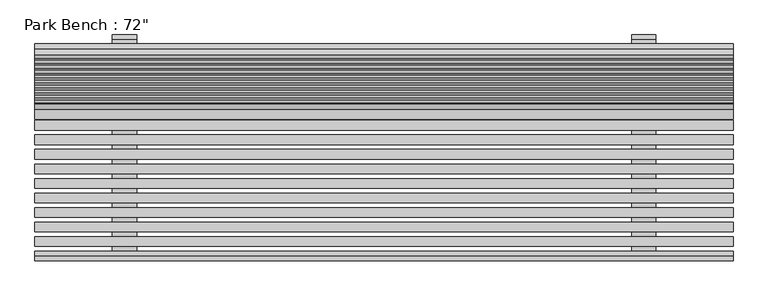
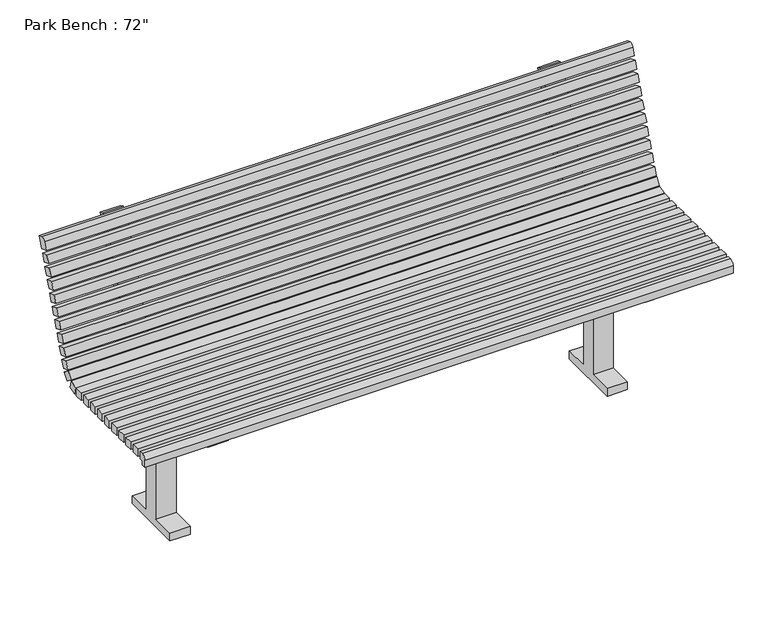
"""IFC4 building model written with IfcOpenShell, lengths in millimetres: geographic element geometry."""

from ifc_helpers import new_model, si_unit, point, frame, frame_2d, origin, place, context, project, spatial, polyline, circle_curve, trimmed, segment, composite_curve, outline, extrude, source, transform, mapped, element, save


def geographic_element_235d1464(model_context):
    return source(origin(), model_context, "Body", "SweptSolid", [
        extrude(outline(polyline([(914.4, -255.4337104), (914.4, -280.8337104), (-914.4, -280.8337104), (-914.4, -255.4337104), (914.4, -255.4337104)])), frame((0.0, 0.0, 457.2), z_axis=(0.0, 0.0, 1.0), x_axis=(1.0, 0.0, 0.0)), (0.0, 0.0, 1.0), 25.4),
        extrude(outline(polyline([(914.4, -217.3337104), (914.4, -242.7337104), (-914.4, -242.7337104), (-914.4, -217.3337104), (914.4, -217.3337104)])), frame((0.0, 0.0, 457.2), z_axis=(0.0, 0.0, 1.0), x_axis=(1.0, 0.0, 0.0)), (0.0, 0.0, 1.0), 25.4),
        extrude(outline(polyline([(914.4, -179.2337104), (914.4, -204.6337104), (-914.4, -204.6337104), (-914.4, -179.2337104), (914.4, -179.2337104)])), frame((0.0, 0.0, 457.2), z_axis=(0.0, 0.0, 1.0), x_axis=(1.0, 0.0, 0.0)), (0.0, 0.0, 1.0), 25.4),
        extrude(outline(polyline([(914.4, -141.1337104), (914.4, -166.5337104), (-914.4, -166.5337104), (-914.4, -141.1337104), (914.4, -141.1337104)])), frame((0.0, 0.0, 457.2), z_axis=(0.0, 0.0, 1.0), x_axis=(1.0, 0.0, 0.0)), (0.0, 0.0, 1.0), 25.4),
        extrude(outline(polyline([(914.4, -103.0337104), (914.4, -128.4337104), (-914.4, -128.4337104), (-914.4, -103.0337104), (914.4, -103.0337104)])), frame((0.0, 0.0, 457.2), z_axis=(0.0, 0.0, 1.0), x_axis=(1.0, 0.0, 0.0)), (0.0, 0.0, 1.0), 25.4),
        extrude(outline(polyline([(914.4, -64.9337104), (914.4, -90.3337104), (-914.4, -90.3337104), (-914.4, -64.9337104), (914.4, -64.9337104)])), frame((0.0, 0.0, 457.2), z_axis=(0.0, 0.0, 1.0), x_axis=(1.0, 0.0, 0.0)), (0.0, 0.0, 1.0), 25.4),
        extrude(outline(polyline([(914.4, -26.8337104), (914.4, -52.2337104), (-914.4, -52.2337104), (-914.4, -26.8337104), (914.4, -26.8337104)])), frame((0.0, 0.0, 457.2), z_axis=(0.0, 0.0, 1.0), x_axis=(1.0, 0.0, 0.0)), (0.0, 0.0, 1.0), 25.4),
        extrude(outline(polyline([(914.4, 11.2662896), (914.4, -14.1337104), (-914.4, -14.1337104), (-914.4, 11.2662896), (914.4, 11.2662896)])), frame((0.0, 0.0, 457.2), z_axis=(0.0, 0.0, 1.0), x_axis=(1.0, 0.0, 0.0)), (0.0, 0.0, 1.0), 25.4),
        extrude(outline(polyline([(914.4, 49.3662896), (914.4, 23.9662896), (-914.4, 23.9662896), (-914.4, 49.3662896), (914.4, 49.3662896)])), frame((0.0, 0.0, 457.2), z_axis=(0.0, 0.0, 1.0), x_axis=(1.0, 0.0, 0.0)), (0.0, 0.0, 1.0), 25.4),
        extrude(outline(composite_curve([segment(polyline([(-304.8, 457.2), (-304.8, 444.5), (-318.9337104, 444.5), (-318.9337104, 468.3125)]), True, "CONTINUOUS"), segment(trimmed(circle_curve(frame_2d((-304.6462104, 468.3125)), 14.2875), [point((-318.9337104, 468.3125))], [point((-304.6462104, 482.6))], False, "CARTESIAN"), True, "CONTINUOUS"), segment(polyline([(-304.6462104, 482.6), (-293.5337104, 482.6), (-293.5337104, 457.2), (-304.8, 457.2)]), True, "CONTINUOUS")], self_intersect=False)), frame((-914.4, 0.0, 0.0), z_axis=(1.0, 0.0, 0.0), x_axis=(0.0, 1.0, 0.0)), (0.0, 0.0, 1.0), 1828.8),
        extrude(outline(polyline([(0.0, -25.4), (0.0, 0.0), (1828.8, 0.0), (1828.8, -25.4), (0.0, -25.4)])), frame((914.4, 121.2738625, 585.5181247), z_axis=(0.0, 0.342020143325687, 0.9396926207859018), x_axis=(-1.0, 0.0, 0.0)), (0.0, 0.0, 1.0), 25.4),
        extrude(outline(polyline([(0.0, -25.4), (0.0, 0.0), (1828.8, 0.0), (1828.8, -25.4), (0.0, -25.4)])), frame((914.4, 134.30483, 621.3204136), z_axis=(0.0, 0.34202014332568254, 0.9396926207859034), x_axis=(-1.0, 0.0, 0.0)), (0.0, 0.0, 1.0), 25.4),
        extrude(outline(polyline([(0.0, -25.3999999), (0.0, 0.0), (1828.8, 0.0), (1828.8, -25.3999999), (0.0, -25.3999999)])), frame((914.4, 95.2119276, 513.913547), z_axis=(0.0, 0.34202014332568254, 0.9396926207859034), x_axis=(-1.0, 0.0, 0.0)), (0.0, 0.0, 1.0), 25.4),
        extrude(outline(polyline([(0.0, -25.4000001), (0.0, 0.0), (1828.8, 0.0), (1828.8, -25.4000001), (0.0, -25.4000001)])), frame((914.4, 108.242895, 549.7158359), z_axis=(0.0, 0.34202014332567804, 0.9396926207859051), x_axis=(-1.0, 0.0, 0.0)), (0.0, 0.0, 1.0), 25.4),
        extrude(outline(polyline([(0.0, -25.4), (0.0, 0.0), (1828.8, 0.0), (1828.8, -25.4), (0.0, -25.4)])), frame((914.4, 173.3977323, 728.7272801), z_axis=(0.0, 0.34202014332568337, 0.9396926207859031), x_axis=(-1.0, 0.0, 0.0)), (0.0, 0.0, 1.0), 25.4),
        extrude(outline(polyline([(0.0, -25.4000001), (0.0, 0.0), (1828.8, 0.0), (1828.8, -25.4000001), (0.0, -25.4000001)])), frame((914.4, 186.4286998, 764.529569), z_axis=(0.0, 0.3420201433256829, 0.9396926207859032), x_axis=(-1.0, 0.0, 0.0)), (0.0, 0.0, 1.0), 25.4),
        extrude(outline(polyline([(0.0, -25.4), (0.0, 0.0), (1828.8, 0.0), (1828.8, -25.4), (0.0, -25.4)])), frame((914.4, 147.3357974, 657.1227024), z_axis=(0.0, 0.3420201433256776, 0.9396926207859052), x_axis=(-1.0, 0.0, 0.0)), (0.0, 0.0, 1.0), 25.4),
        extrude(outline(polyline([(0.0, -25.4), (0.0, 0.0), (1828.8, 0.0), (1828.8, -25.4), (0.0, -25.4)])), frame((914.4, 160.3667649, 692.9249913), z_axis=(0.0, 0.34202014332568254, 0.9396926207859034), x_axis=(-1.0, 0.0, 0.0)), (0.0, 0.0, 1.0), 25.4),
        extrude(outline(polyline([(0.0, -25.3999999), (0.0, 0.0), (1828.8, 0.0), (1828.8, -25.3999999), (0.0, -25.3999999)])), frame((914.4, 199.4596673, 800.3318578), z_axis=(0.0, 0.3420201433256774, 0.9396926207859052), x_axis=(-1.0, 0.0, 0.0)), (0.0, 0.0, 1.0), 25.4),
        extrude(outline(composite_curve([segment(polyline([(249.3897948, 863.2491239), (236.3588273, 827.4468351), (212.4906347, 836.1341467), (221.1779464, 860.0023393)]), True, "CONTINUOUS"), segment(trimmed(circle_curve(frame_2d((233.1120426, 855.6586834)), 12.7), [point((221.1779464, 860.0023393))], [point((237.4556985, 867.5927797))], False, "CARTESIAN"), True, "CONTINUOUS"), segment(polyline([(237.4556985, 867.5927797), (249.3897948, 863.2491239)]), True, "CONTINUOUS")], self_intersect=False)), frame((-914.4, 0.0, 0.0), z_axis=(1.0, 0.0, 0.0), x_axis=(0.0, 1.0, 0.0)), (0.0, 0.0, 1.0), 1828.8),
        extrude(outline(polyline([(0.0, -25.4), (0.0, 0.0), (1828.8, 0.0), (1828.8, -25.4), (0.0, -25.4)])), frame((914.4, 78.7855779, 490.7267336), z_axis=(0.0, 0.5735764363510742, 0.8191520442889721), x_axis=(-1.0, 0.0, 0.0)), (0.0, 0.0, 1.0), 25.4),
        extrude(outline(polyline([(0.0, -25.4), (0.0, 0.0), (1828.8, 0.0), (1828.8, -25.4), (0.0, -25.4)])), frame((914.4, 59.0817015, 457.2297909), z_axis=(0.0, -0.2588190451024684, 0.9659258262890824), x_axis=(-1.0, 0.0, 0.0)), (0.0, 0.0, 1.0), 25.4),
        extrude(outline(composite_curve([segment(polyline([(-101.6, 25.4), (-25.4, 25.4), (-25.4, 431.8), (-304.8, 431.8), (-304.8, 457.2), (57.1368213, 457.2)]), True, "CONTINUOUS"), segment(trimmed(circle_curve(frame_2d((57.1368213, 520.7)), 63.5), [point((57.1368213, 457.2))], [point((116.8073027, 498.9817209))], True, "CARTESIAN"), True, "CONTINUOUS"), segment(polyline([(116.8073027, 498.9817209), (244.9406421, 851.0251774)]), True, "CONTINUOUS"), segment(trimmed(circle_curve(frame_2d((256.8747384, 846.6815216)), 12.7), [point((244.9406421, 851.0251774))], [point((261.2183942, 858.6156178))], False, "CARTESIAN"), True, "CONTINUOUS"), segment(polyline([(261.2183942, 858.6156178), (273.1524905, 854.271962), (140.6754953, 490.2944093)]), True, "CONTINUOUS"), segment(trimmed(circle_curve(frame_2d((57.1368213, 520.7)), 88.9), [point((140.6754953, 490.2944093))], [point((57.1368213, 431.8))], False, "CARTESIAN"), True, "CONTINUOUS"), segment(polyline([(57.1368213, 431.8), (25.4, 431.8), (25.4, 25.4), (101.6, 25.4), (101.6, 0.0), (-101.6, 0.0), (-101.6, 25.4)]), True, "CONTINUOUS")], self_intersect=False)), frame((648.3736591, 0.0, 0.0), z_axis=(1.0, 0.0, 0.0), x_axis=(0.0, 1.0, 0.0)), (0.0, 0.0, 1.0), 62.8263409),
        extrude(outline(composite_curve([segment(polyline([(-101.6, 25.4), (-25.4, 25.4), (-25.4, 431.8), (-304.8, 431.8), (-304.8, 457.2), (57.1368213, 457.2)]), True, "CONTINUOUS"), segment(trimmed(circle_curve(frame_2d((57.1368213, 520.7)), 63.5), [point((57.1368213, 457.2))], [point((116.8073027, 498.9817209))], True, "CARTESIAN"), True, "CONTINUOUS"), segment(polyline([(116.8073027, 498.9817209), (244.9406421, 851.0251774)]), True, "CONTINUOUS"), segment(trimmed(circle_curve(frame_2d((256.8747384, 846.6815216)), 12.7), [point((244.9406421, 851.0251774))], [point((261.2183942, 858.6156178))], False, "CARTESIAN"), True, "CONTINUOUS"), segment(polyline([(261.2183942, 858.6156178), (273.1524905, 854.271962), (140.6754953, 490.2944093)]), True, "CONTINUOUS"), segment(trimmed(circle_curve(frame_2d((57.1368213, 520.7)), 88.9), [point((140.6754953, 490.2944093))], [point((57.1368213, 431.8))], False, "CARTESIAN"), True, "CONTINUOUS"), segment(polyline([(57.1368213, 431.8), (25.4, 431.8), (25.4, 25.4), (101.6, 25.4), (101.6, 0.0), (-101.6, 0.0), (-101.6, 25.4)]), True, "CONTINUOUS")], self_intersect=False)), frame((-711.2, 0.0, 0.0), z_axis=(1.0, 0.0, 0.0), x_axis=(0.0, 1.0, 0.0)), (0.0, 0.0, 1.0), 63.8916859),
    ])


if __name__ == "__main__":
    model = new_model("IFC4")
    model_context = context("Model", 3, world=origin())
    ifc_project = project(units=[si_unit("LENGTHUNIT", "METRE", prefix="MILLI")], contexts=[model_context])
    site = spatial("IfcSite", under=ifc_project)
    building = spatial("IfcBuilding", under=site)
    placement = place(None, origin())
    geographic_element_shape = geographic_element_235d1464(model_context)
    element("IfcGeographicElement", 1, ObjectType="Park Bench : 72\"", at=placement, inside=building, context=model_context, shape_type="MappedRepresentation", body=[
        mapped(geographic_element_shape, transform((0.0, 0.0, 0.0), x_axis=(1.0, 0.0, 0.0), y_axis=(0.0, 1.0, 0.0), z_axis=(0.0, 0.0, 1.0))),
    ])
    save(model, "model.ifc")

# Revit data of these elements
# Type "Park Bench : 72\""
#   Length = 6' - 0"
#   Seat Material = Wood - Teak
#   Frame Material = Steel, Paint Finish, Dark Gray, Matte
# Element 1 (IfcGeographicElement, "Park Bench : 72\"")
#   Materials on its faces: "Wood - Teak", "Steel, Paint Finish, Dark Gray, Matte"
# Materials
#   "Wood - Teak": class "Wood", colour RGB 145 112 90, transparency 0
#   "Steel, Paint Finish, Dark Gray, Matte": class "Metal", colour RGB 98 98 98, transparency 0, Description = "Steel, paint finish, dark gray, matte", Cost = 0
